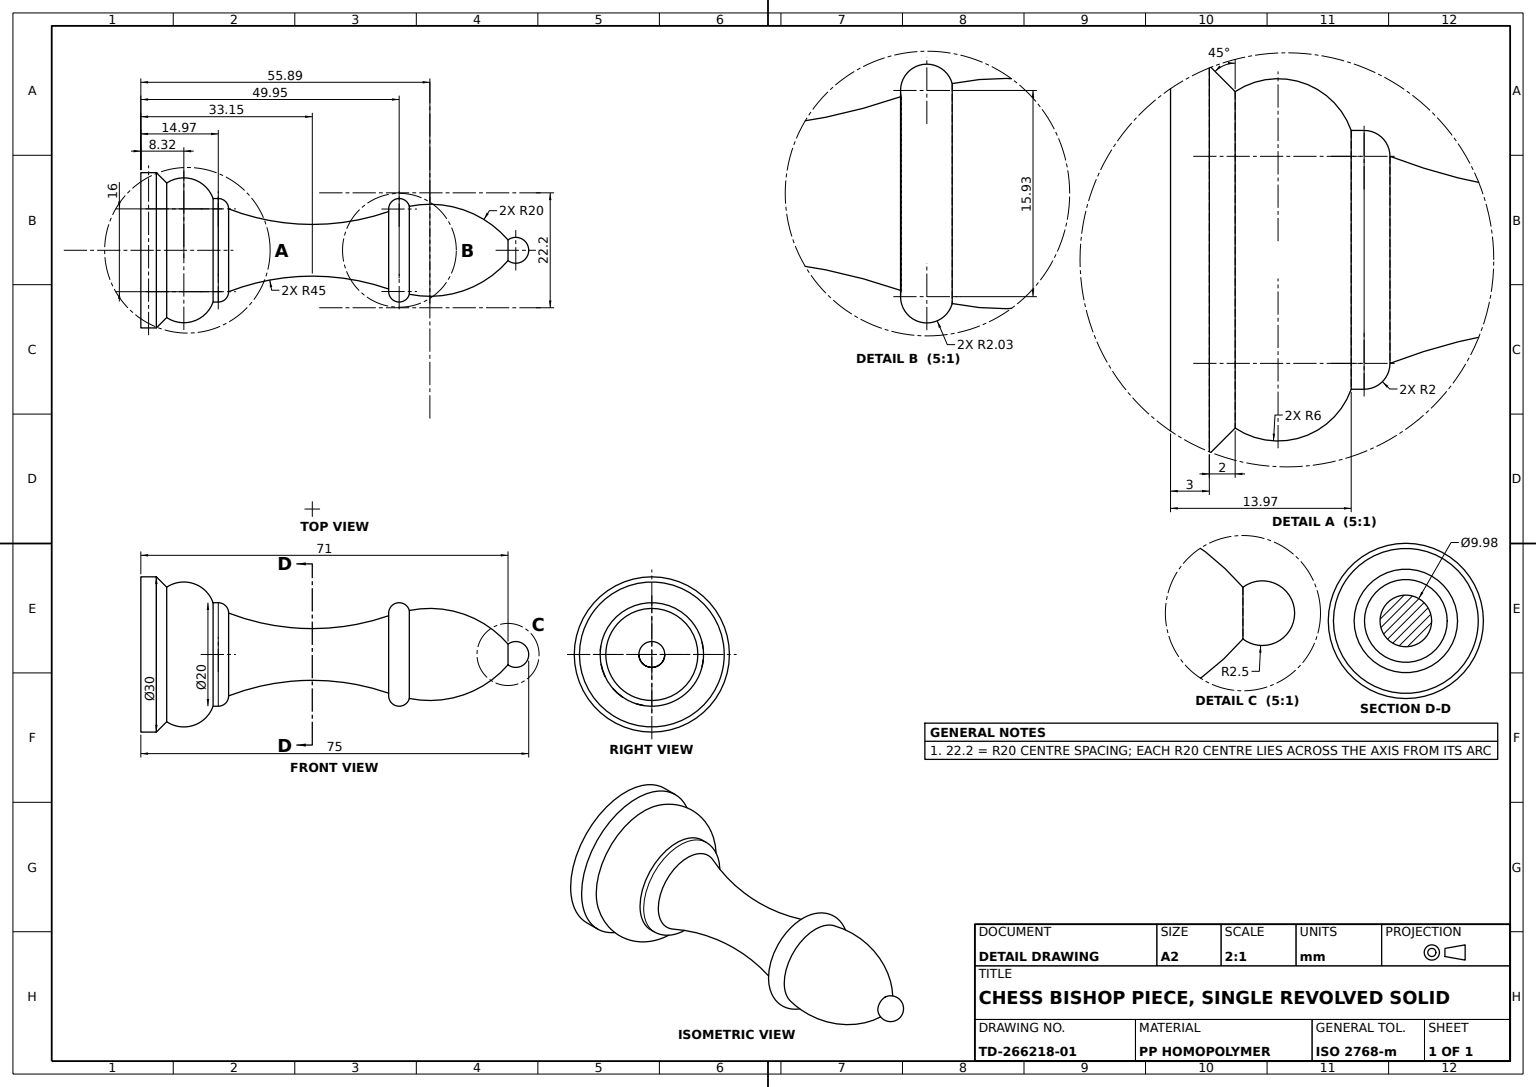
SolidWorks part; units mm, degrees
material "PP Homopolymer"
ref_plane "Front Plane" through (0, 0, 0) normal (0, 0, 1) x (1, 0, 0)
ref_plane "Top Plane" through (0, 0, 0) normal (0, 1, 0) x (1, 0, 0)
ref_plane "Right Plane" through (0, 0, 0) normal (1, 0, 0) x (0, 0, -1)
sketch "Bishop Profile Sketch" plane through (0, 0, 0) normal (0, 0, 1) x (1, 0, 0)
  line L0 (0, 0) -> (0, 75)
  line L1 (0, 0) -> (15, 0)
  line L2 (15, 0) -> (15, 3)
  line L3 (15, 3) -> (13, 5)
  line L4 (10, 13.9735) -> (10, 14.9735)
  line L5 (2.5, 75) -> (2.5, 71.546) construction
  line L6 (10, 61.8501) -> (10, 46.791) construction
  line L7 (14, 13.3001) -> (14, -1.935) construction
  arc A1 (10, 14.9735) -> (8, 16.9735) centre (8, 14.9735) ccw
  arc A2 (8, 16.9735) -> (7.5, 47.9735) centre (49.9901, 33.1548) cw
  arc A3 (7.5, 47.9735) -> (8.5, 51.9135) centre (7.9673, 49.9518) ccw
  arc A4 (8.5, 51.9135) -> (2, 71) centre (-11.101, 55.8883) ccw
  arc A5 (2, 71) -> (0, 75) centre (0, 72.5) ccw
  arc A6 (10, 13.9735) -> (13, 5) centre (8, 8.3166) cw
  dimension "D4" = 2
  dimension "D8" = 2
  dimension "D9" = 45
  dimension "D16" = 20
  dimension "D20" = 6
  dimension "D21" = 3.94
  dimension "D1" = 75
  dimension "D2" = 15
  dimension "D3" = 13
  dimension "D5" = 14
  dimension "D6" = 1
  dimension "D7" = 2
  dimension "D10" = 31
  dimension "D11" = 10
  dimension "D12" = 7.5
  dimension "D13" = 8.5
  dimension "D14" = 10
  dimension "D15" = 2
  dimension "D17" = 4
  dimension "D18" = 2.5
  dimension "D19" = 3
revolve "Bishop Body Revolve" add sketch "Bishop Profile Sketch" angle 360 about L0
